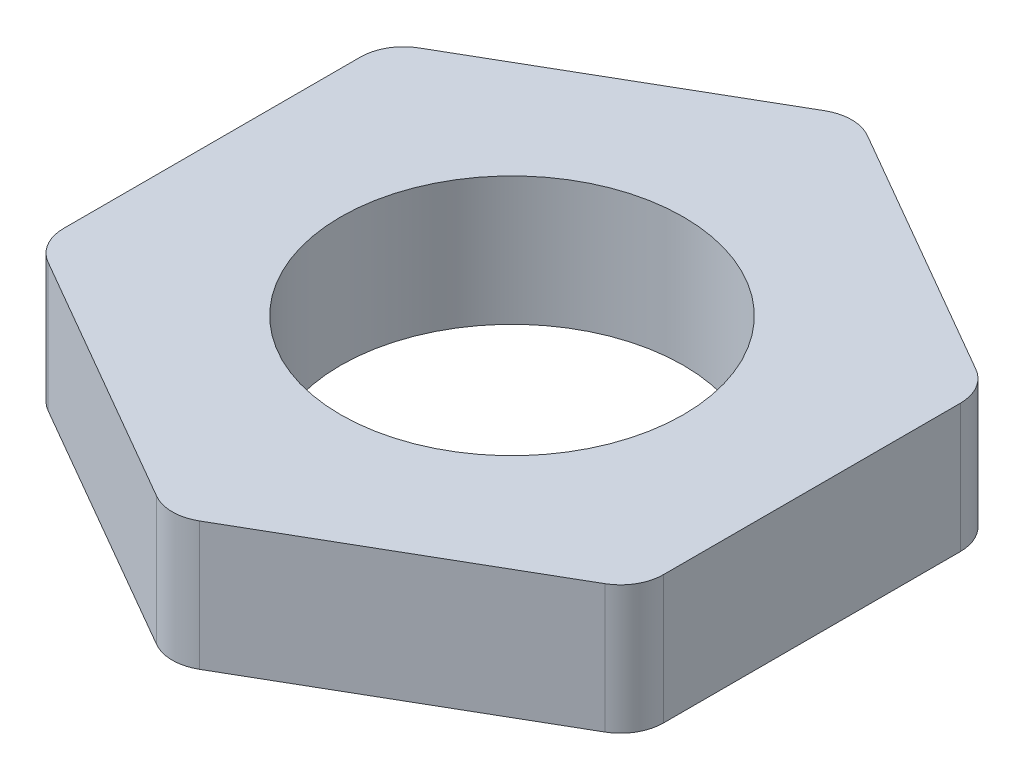
SolidWorks part; units mm, degrees
material "Plain Carbon Steel"
ref_plane "Front Plane" through (0, 0, 0) normal (0, 0, 1) x (1, 0, 0)
ref_plane "Top Plane" through (0, 0, 0) normal (0, 1, 0) x (1, 0, 0)
ref_plane "Right Plane" through (0, 0, 0) normal (1, 0, 0) x (0, 0, -1)
sketch "Hex Profile 14AF" plane through (0, 0, 0) normal (0, 1, 0) x (1, 0, 0)
  line L0 (-158.8374, 0) -> (7783.0331, 0) construction
  line L1 (0, -158.8374) -> (0, 7783.0331) construction
  line L3 (0, 8.0829) -> (-7, 4.0415)
  line L4 (-7, 4.0415) -> (-7, -4.0415)
  line L5 (-7, -4.0415) -> (0, -8.0829)
  line L6 (0, -8.0829) -> (7, -4.0415)
  line L7 (7, -4.0415) -> (7, 4.0415)
  line L8 (7, 4.0415) -> (0, 8.0829)
  circle A0 centre (0, 0) radius 7 construction
  dimension "D1" = 14
extrude "Hex Body 3mm" add sketch "Hex Profile 14AF" along normal blind 3
sketch "Bore Profile Ø8" plane through (0, 3, 0) normal (0, 1, 0) x (1, 0, 0)
  circle A0 centre (0, 0) radius 4
  dimension "D1" = 8
extrude "Bore Ø8" cut sketch "Bore Profile Ø8" against normal blind 3
fillet "Hex Corner Fillets R1" radius 1 6 edges at (-7, 1.5, 4.0415) (-7, 1.5, -4.0415) (0, 1.5, -8.0829) (7, 1.5, -4.0415) (7, 1.5, 4.0415) (0, 1.5, 8.0829)
